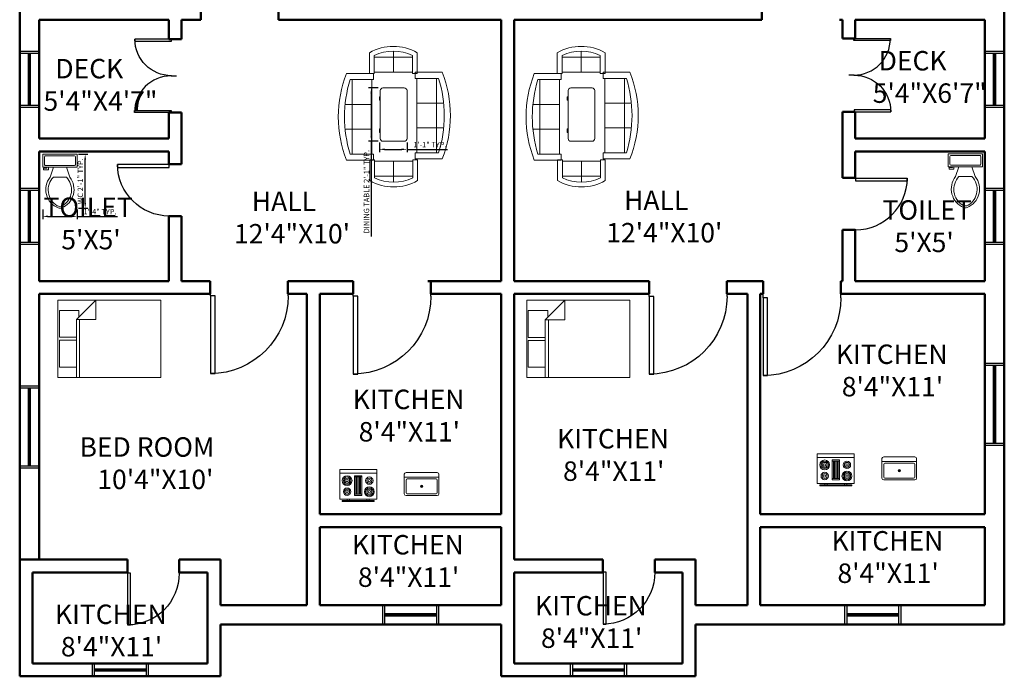
# Model space of a CAD drawing. Units: inches. Extents: x -31438 to -28352, y 12489 to 13610.
# Tile 4 of 5: x -29143 to -28687, y 12722 to 13026. Entities that reach past the tile are written whole.
import ezdxf

# ---------------------------------------------------------------- set-up
doc = ezdxf.new("R2010")
doc.units = ezdxf.units.IN
for name, color, linetype, lineweight in [('A-ANNO-DIMS', 2, 'Continuous', 18), ('A-AREA-IDEN', 3, 'Continuous', 18), ('A-DOOR', 3, 'Continuous', 25), ('A-FLOR-FIXT', 9, 'Continuous', 18), ('A-FURN', 8, 'Continuous', 18), ('A-GLAZ', 4, 'Continuous', 25), ('A-WALL', 7, 'Continuous', 50)]:
    doc.layers.add(name, color=color, linetype=linetype, lineweight=lineweight)
doc.styles.get("Standard").update_dxf_attribs({"font": 'arial.ttf'})
doc.dimstyles.new('ISO-25', dxfattribs={"dimtxt": 2.5, "dimasz": 2.5, "dimexe": 1.25, "dimexo": 0.625, "dimtad": 1, "dimdec": 0, "dimlunit": 3, "dimtxsty": 'Standard', "dimcen": 2.5, "dimadec": 0, "dimazin": 0, "dimtfac": 1, "dimtdec": 0, "dimtmove": 0, "dimatfit": 3, "dimfxl": 1, "dimarcsym": 0})

# ---------------------------------------------------------------- blocks, each defined once
blk = doc.blocks.new('*U8')
for p, q in [((0, 0), (0, -100)), ((750, 0), (750, -100))]:
    blk.add_line(p, q)
blk.add_lwpolyline([(0, 0), (0, 750), (43.75, 750), (43.75, 0)], close=True)
blk.add_arc((0, 0), 750, 0, 90)
blk = doc.blocks.new('Bed - Queen')
for p, q in [((0, -80.00003), (0, 0)), ((0, 0), (59.99999, 0)), ((59.99999, 0), (59.99999, -80.00003)), ((7.99999, -1.2), (28.79998, -1.2)), ((7.99999, -14.4), (7.99999, -1.2)), ((28.79998, -1.2), (28.79998, -14.4)), ((31.19999, -1.2), (51.99999, -1.2)), ((31.19999, -14.4), (31.19999, -1.2)), ((51.99999, -1.2), (51.99999, -16.4)), ((0, -14.4), (44.8, -14.4)), ((59.99999, -29.6), (44.8, -14.4)), ((44.8, -14.4), (44.8, -29.6)), ((44.8, -16.8), (0, -16.8)), ((51.99999, -16.4), (46.79936, -16.4)), ((44.8, -29.6), (59.99999, -29.6)), ((59.99999, -80.00003), (0, -80.00003))]:
    blk.add_line(p, q)
blk = doc.blocks.new('Desk - 30 x 60 in.')
for p, q in [((-26.999995, 0), (26.999995, 0)), ((-29.999995, -27), (-29.999995, -3)), ((29.999995, -3), (29.999995, -27)), ((26.999995, -30), (-26.999995, -30)), ((-20.000005, -30), (-20.000005, -31)), ((-20.000005, -31), (-16.000005, -31)), ((-16.000005, -31), (-16.000005, -30)), ((15.999995, -31), (15.999995, -30)), ((19.999995, -31), (15.999995, -31)), ((19.999995, -30), (19.999995, -31))]:
    blk.add_line(p, q)
for centre, start, end in [((-26.499995, -3.5), 98.1301, 171.8699), ((26.499995, -3.5), 8.130102, 81.8699), ((-26.499995, -26.5), 188.1301, 261.8699), ((26.499995, -26.5), 278.1301, 351.8699)]:
    blk.add_arc(centre, 3.535534, start, end)
blk = doc.blocks.new('Sofa - Roundback 7 ft.')
for p, q in [((-12.00002, -32.4421), (-12.00003, -6.5971)), ((11.99997, -32.4421), (11.99998, -6.5971)), ((-36.000027, -34), (-36.000027, -11.4696)), ((-35.999844, -13.3819), (35.9998, -13.3819)), ((35.99998, -34), (35.99998, -11.4696)), ((-36.000027, -32.4421), (35.99998, -32.4421))]:
    blk.add_line(p, q)
for points in [[(-36.000027, -34), (-42.000027, -34), (-42.000027, -8)], [(41.99998, -8), (41.99998, -34), (35.99998, -34)]]:
    blk.add_lwpolyline(points)
for centre, radius, start, end in [((0, -114.25), 114.25, 68.43141, 111.5686), ((-0.00001, -127.1968), 121.1968, 72.72033, 107.2797)]:
    blk.add_arc(centre, radius, start, end)
blk = doc.blocks.new('Sofa - Roundback Loveseat 5 ft.')
for p, q in [((-24, -33.99998), (-24, -11.46958)), ((0, -32.44198), (0, -5.99998)), ((24.00004, -33.99998), (24.00004, -11.46958)), ((-23.9998, -13.38178), (23.99986, -13.38178)), ((-24, -32.44198), (24.00004, -32.44198))]:
    blk.add_line(p, q)
for points in [[(-24, -33.99998), (-30, -33.99998), (-30, -7.99998)], [(30.00004, -7.99998), (30.00004, -33.99998), (24.00004, -33.99998)]]:
    blk.add_lwpolyline(points)
for centre, radius, start, end in [((0, -60.24998), 60.24998, 60.13715, 119.8628), ((0, -61.38438), 55.38444, 64.32083, 115.6792)]:
    blk.add_arc(centre, radius, start, end)
blk = doc.blocks.new('Toilet - top')
for p, q in [((9.5, -6), (9.5, -2)), ((-10, -8.5), (-8, -8.5)), ((-10, -9.5), (-10, -8.5)), ((-7, -9.5), (-10, -9.5)), ((-8, -8.5), (-8, -8)), ((-7, -8), (-7, -9.5)), ((-4, -8), (-6, -14)), ((4, -8), (6, -14)), ((4, -14), (-4, -14))]:
    blk.add_line(p, q)
blk.add_lwpolyline([(10.5, -8), (10.5, 0), (-10.5, 0), (-10.5, -8)], close=True)
for points in [[(-9.5, -2), (-9.5, -6)], [(8.5, -1), (-8.5, -1)], [(-8.5, -7), (8.5, -7)]]:
    blk.add_lwpolyline(points)
for centre, radius, start, end in [((-8.62, -1.88), 0.884, 81.8699, 188.1301), ((-8.62, -6.12), 0.884, 171.8699, 278.1301), ((8.62, -1.88), 0.884, 351.8699, 98.1301), ((8.62, -6.12), 0.884, 261.8699, 8.1301), ((3.52, -21.58), 12.17, 141.46911, 247.97143), ((4.2, -21.82), 11.33, 136.36773, 238.94682), ((-3.52, -21.58), 12.17, 292.02843, 38.53071), ((-4.2, -21.82), 11.33, 301.05301, 43.63209), ((0, -27.88), 4, 245.73182, 294.26817), ((0, -29), 4, 254.86053, 285.13947)]:
    blk.add_arc(centre, radius, start, end)
blk = doc.blocks.new('Range-Oven - 30 in top')
for p, q in [((0, -3), (30, -3)), ((12, -6), (18, -6)), ((13, -20), (13, -6)), ((14, -6), (14, -20)), ((15, -20), (15, -6)), ((16, -6), (16, -20)), ((17, -20), (17, -6)), ((18, -20), (12, -20)), ((6, -24), (6, -25)), ((8, -25), (8, -24)), ((22, -25), (22, -24)), ((24, -24), (24, -25))]:
    blk.add_line(p, q)
for points in [[(0, -24), (0, 0), (30, 0), (30, -24)], [(12, -21), (12, -5), (18, -5), (18, -21)], [(2, -26), (2, -25), (28, -25), (28, -26)]]:
    blk.add_lwpolyline(points, close=True)
for centre, radius in [((6, -9), 4), ((6, -9), 3), ((6, -9), 2), ((24, -9), 3), ((24, -9), 2), ((6, -18), 3), ((6, -9), 1), ((24, -18), 4), ((24, -18), 3), ((24, -9), 1), ((6, -18), 2), ((6, -18), 1), ((24, -18), 2), ((24, -18), 1)]:
    blk.add_circle(centre, radius)
blk = doc.blocks.new('Sink-single - 30 in top')
blk.add_line((-15, -3.999996), (15, -3.999996))
for points in [[(-13.5, 0), (13.5, 0)], [(-15, -18.499996), (-15, -1.5)], [(-13.5, -17.499996), (-13.5, -6.499996)], [(-12.5, -5.499996), (12.5, -5.499996)], [(13.5, -6.499996), (13.5, -17.499996)], [(15, -1.5), (15, -18.499996)], [(13.5, -19.999996), (-13.5, -19.999996)], [(12.5, -18.499996), (-12.5, -18.499996)]]:
    blk.add_lwpolyline(points)
for radius in [1, 0.5]:
    blk.add_circle((0, -11.999996), radius)
for centre, radius, start, end in [((-13.5, -1.5), 1.5, 90, 180), ((-12.5, -6.499996), 1, 90, 180), ((12.5, -6.499996), 1, 0, 90), ((13.5, -1.5), 1.5, 0, 90), ((-13.5, -18.499996), 1.5, 180, 270), ((-12.5, -17.499996), 1, 180, 270), ((12.5, -17.499996), 1, 270, 0), ((13.5, -18.499996), 1.5, 270, 0)]:
    blk.add_arc(centre, radius, start, end)
blk = doc.blocks.new('WIN-24')
for p, q in [((0, 0), (0, 24)), ((0.5, 0), (0.5, 24))]:
    blk.add_line(p, q)
blk = doc.blocks.new('*D191')
at = {"layer": 'A-ANNO-DIMS', "color": 0, "lineweight": -2, "transparency": 16777216}
for p, q in [((-29115.8, 12963.47), (-29111.42, 12963.47)), ((-29112.67, 12940.94), (-29112.67, 12960.97)), ((-29115.8, 12938.44), (-29111.42, 12938.44))]:
    blk.add_line(p, q, dxfattribs=at)
at = {"layer": 'A-ANNO-DIMS', "color": 0, "transparency": 16777216}
for points in [[(-29113.09, 12960.97), (-29112.25, 12960.97), (-29112.67, 12963.47)], [(-29113.09, 12940.94), (-29112.25, 12940.94), (-29112.67, 12938.44)]]:
    blk.add_solid(points, dxfattribs=at)
at = {"layer": 'Defpoints', "color": 0, "transparency": 16777216}
for p in [(-29116.42, 12963.47), (-29112.67, 12963.47), (-29116.42, 12938.44)]:
    blk.add_point(p, dxfattribs=at)
at = {"layer": 'A-ANNO-DIMS', "color": 0, "transparency": 16777216, "insert": (-29114.59, 12950.96), "char_height": 2.5, "attachment_point": 5, "rotation": 90}
blk.add_mtext('WC 2\'-1" TYP.', dxfattribs=at)
blk = doc.blocks.new('*D192')
at = {"layer": 'A-ANNO-DIMS', "color": 0, "lineweight": -2, "transparency": 16777216}
for p, q in [((-29132.33, 12937.81), (-29132.33, 12933.43)), ((-29116.42, 12937.81), (-29116.42, 12933.43)), ((-29129.83, 12934.68), (-29118.92, 12934.68)), ((-29116.42, 12934.68), (-29097.67, 12934.68))]:
    blk.add_line(p, q, dxfattribs=at)
at = {"layer": 'A-ANNO-DIMS', "color": 0, "transparency": 16777216}
for points in [[(-29129.83, 12935.1), (-29129.83, 12934.27), (-29132.33, 12934.68)], [(-29118.92, 12935.1), (-29118.92, 12934.27), (-29116.42, 12934.68)]]:
    blk.add_solid(points, dxfattribs=at)
at = {"layer": 'Defpoints', "color": 0, "transparency": 16777216}
for p in [(-29132.33, 12938.44), (-29116.42, 12938.44), (-29116.42, 12934.68)]:
    blk.add_point(p, dxfattribs=at)
at = {"layer": 'A-ANNO-DIMS', "color": 0, "transparency": 16777216, "insert": (-29105.8, 12936.56), "char_height": 2.5, "attachment_point": 5}
blk.add_mtext('1\'-4" TYP.', dxfattribs=at)
blk = doc.blocks.new('*D203')
at = {"layer": 'A-ANNO-DIMS', "color": 0, "lineweight": -2, "transparency": 16777216}
for p, q in [((-28977.05, 12994.22), (-28981.39, 12994.22)), ((-28980.14, 12991.72), (-28980.14, 12971.94)), ((-28977.05, 12969.44), (-28981.39, 12969.44)), ((-28980.14, 12969.44), (-28980.14, 12925.35))]:
    blk.add_line(p, q, dxfattribs=at)
at = {"layer": 'A-ANNO-DIMS', "color": 0, "transparency": 16777216}
for points in [[(-28980.56, 12991.72), (-28979.72, 12991.72), (-28980.14, 12994.22)], [(-28980.56, 12971.94), (-28979.72, 12971.94), (-28980.14, 12969.44)]]:
    blk.add_solid(points, dxfattribs=at)
at = {"layer": 'Defpoints', "color": 0, "transparency": 16777216}
for p in [(-28976.42, 12994.22), (-28980.14, 12969.44), (-28976.42, 12969.44)]:
    blk.add_point(p, dxfattribs=at)
at = {"layer": 'A-ANNO-DIMS', "color": 0, "transparency": 16777216, "insert": (-28982.06, 12946.15), "char_height": 2.5, "attachment_point": 5, "rotation": 90}
blk.add_mtext('DINING TABLE 2\'-1" TYP.', dxfattribs=at)
blk = doc.blocks.new('*D204')
at = {"layer": 'A-ANNO-DIMS', "color": 0, "lineweight": -2, "transparency": 16777216}
for p, q in [((-28976.42, 12968.82), (-28976.42, 12964.47)), ((-28963.62, 12968.82), (-28963.62, 12964.47)), ((-28973.92, 12965.72), (-28966.12, 12965.72)), ((-28963.62, 12965.72), (-28944.87, 12965.72))]:
    blk.add_line(p, q, dxfattribs=at)
at = {"layer": 'A-ANNO-DIMS', "color": 0, "transparency": 16777216}
for points in [[(-28973.92, 12966.14), (-28973.92, 12965.31), (-28976.42, 12965.72)], [(-28966.12, 12966.14), (-28966.12, 12965.31), (-28963.62, 12965.72)]]:
    blk.add_solid(points, dxfattribs=at)
at = {"layer": 'Defpoints', "color": 0, "transparency": 16777216}
for p in [(-28976.42, 12969.44), (-28963.62, 12969.44), (-28963.62, 12965.72)]:
    blk.add_point(p, dxfattribs=at)
at = {"layer": 'A-ANNO-DIMS', "color": 0, "transparency": 16777216, "insert": (-28952.99, 12967.61), "char_height": 2.5, "attachment_point": 5}
blk.add_mtext('1\'-1" TYP.', dxfattribs=at)

msp = doc.modelspace()

# ---------------------------------------------------------------- linework, layer by layer
at = {"layer": 'A-GLAZ'}
for p, q in [((-29142.99, 13011.25), (-29133.99, 13011.25)), ((-29142.99, 13010.25), (-29133.99, 13010.25)), ((-29138.99, 12986.25), (-29138.99, 13010.25)), ((-29138.49, 12986.25), (-29138.49, 13010.25)), ((-29137.99, 12986.25), (-29137.99, 13010.25)), ((-28695.99, 13011.25), (-28686.99, 13011.25)), ((-28695.99, 13010.25), (-28686.99, 13010.25)), ((-28691.99, 12986.25), (-28691.99, 13010.25)), ((-28691.49, 12986.25), (-28691.49, 13010.25)), ((-28690.99, 12986.25), (-28690.99, 13010.25)), ((-29142.99, 12986.25), (-29133.99, 12986.25)), ((-29142.99, 12985.25), (-29133.99, 12985.25)), ((-28695.99, 12986.25), (-28686.99, 12986.25)), ((-28695.99, 12985.25), (-28686.99, 12985.25)), ((-29142.99, 12947.75), (-29133.99, 12947.75)), ((-29142.99, 12946.75), (-29133.99, 12946.75)), ((-29138.99, 12922.75), (-29138.99, 12946.75)), ((-29138.49, 12922.75), (-29138.49, 12946.75)), ((-29137.99, 12922.75), (-29137.99, 12946.75)), ((-28695.99, 12947.75), (-28686.99, 12947.75)), ((-28695.99, 12946.75), (-28686.99, 12946.75)), ((-28691.99, 12922.75), (-28691.99, 12946.75)), ((-28691.49, 12922.75), (-28691.49, 12946.75)), ((-28690.99, 12922.75), (-28690.99, 12946.75)), ((-29142.99, 12922.75), (-29133.99, 12922.75)), ((-29142.99, 12921.75), (-29133.99, 12921.75)), ((-28695.99, 12922.75), (-28686.99, 12922.75)), ((-28695.99, 12921.75), (-28686.99, 12921.75)), ((-28695.99, 12866.75), (-28686.99, 12866.75)), ((-28695.99, 12865.75), (-28686.99, 12865.75)), ((-28691.99, 12829.75), (-28691.99, 12865.75)), ((-28691.49, 12829.75), (-28691.49, 12865.75)), ((-28690.99, 12829.75), (-28690.99, 12865.75)), ((-29142.99, 12856.25), (-29133.99, 12856.25)), ((-29142.99, 12855.25), (-29133.99, 12855.25)), ((-29138.99, 12819.25), (-29138.99, 12855.25)), ((-29138.49, 12819.25), (-29138.49, 12855.25)), ((-29137.99, 12819.25), (-29137.99, 12855.25)), ((-28695.99, 12829.75), (-28686.99, 12829.75)), ((-28695.99, 12828.75), (-28686.99, 12828.75)), ((-29142.99, 12819.25), (-29133.99, 12819.25)), ((-29142.99, 12818.25), (-29133.99, 12818.25)), ((-28974.99, 12754.75), (-28974.99, 12745.75)), ((-28973.99, 12754.75), (-28973.99, 12745.75)), ((-28949.99, 12754.75), (-28949.99, 12745.75)), ((-28948.99, 12754.75), (-28948.99, 12745.75)), ((-28760.99, 12754.75), (-28760.99, 12745.75)), ((-28759.99, 12754.75), (-28759.99, 12745.75)), ((-28735.99, 12754.75), (-28735.99, 12745.75)), ((-28734.99, 12754.75), (-28734.99, 12745.75)), ((-28973.99, 12750.75), (-28949.99, 12750.75)), ((-28759.99, 12750.75), (-28735.99, 12750.75)), ((-29109.49, 12727.75), (-29109.49, 12721.75)), ((-29108.49, 12727.75), (-29108.49, 12721.75)), ((-29084.49, 12727.75), (-29084.49, 12721.75)), ((-29083.49, 12727.75), (-29083.49, 12721.75)), ((-28887.99, 12727.75), (-28887.99, 12721.75)), ((-28886.99, 12727.75), (-28886.99, 12721.75)), ((-28862.99, 12727.75), (-28862.99, 12721.75)), ((-28861.99, 12727.75), (-28861.99, 12721.75)), ((-29108.49, 12725.25), (-29084.49, 12725.25)), ((-29108.49, 12724.75), (-29084.49, 12724.75)), ((-29108.49, 12724.25), (-29084.49, 12724.25)), ((-28886.99, 12725.25), (-28862.99, 12725.25)), ((-28886.99, 12724.75), (-28862.99, 12724.75)), ((-28886.99, 12724.25), (-28862.99, 12724.25))]:
    msp.add_line(p, q, dxfattribs=at)
at = {"layer": 'A-WALL'}
for p, q in [((-28686.99, 13609.75), (-28686.99, 12745.75)), ((-29142.99, 12721.75), (-29142.99, 13585.75)), ((-29059.11, 13031.75), (-29059.11, 13025.75)), ((-29023.11, 13031.75), (-29023.11, 13025.75)), ((-28799.32, 13031.75), (-28799.32, 13025.75)), ((-29073.99, 13025.75), (-29133.99, 13025.75)), ((-29133.99, 12970.75), (-29133.99, 13025.75)), ((-29073.99, 13016.72), (-29073.99, 13025.75)), ((-29059.11, 13025.75), (-29067.99, 13025.75)), ((-29067.99, 13016.72), (-29067.99, 13025.75)), ((-28953.99, 13025.75), (-29023.11, 13025.75)), ((-28919.99, 13025.75), (-28953.99, 13025.75)), ((-28919.99, 12904.75), (-28919.99, 13025.75)), ((-28799.32, 13025.75), (-28913.99, 13025.75)), ((-28913.99, 12904.75), (-28913.99, 13025.75)), ((-28761.99, 13025.75), (-28763.32, 13025.75)), ((-28761.99, 13025.75), (-28761.99, 13017.05)), ((-28755.99, 13025.75), (-28755.99, 13017.05)), ((-28695.99, 13025.75), (-28755.99, 13025.75)), ((-28695.99, 13025.75), (-28755.99, 13025.75)), ((-28695.99, 13025.75), (-28695.99, 12970.75)), ((-29073.99, 13016.72), (-29067.99, 13016.72)), ((-28761.99, 13017.05), (-28755.99, 13017.05)), ((-29073.99, 12970.75), (-29073.99, 12982.72)), ((-29073.99, 12982.72), (-29067.99, 12982.72)), ((-29067.99, 12958.83), (-29067.99, 12982.72)), ((-28761.99, 12983.05), (-28761.99, 12952.5)), ((-28761.99, 12983.05), (-28755.99, 12983.05)), ((-28755.99, 12983.05), (-28755.99, 12970.75)), ((-29073.99, 12970.75), (-29133.99, 12970.75)), ((-28695.99, 12970.75), (-28755.99, 12970.75)), ((-28695.99, 12970.75), (-28755.99, 12970.75)), ((-29073.99, 12964.75), (-29133.99, 12964.75)), ((-29133.99, 12904.75), (-29133.99, 12964.75)), ((-29073.99, 12958.83), (-29073.99, 12964.75)), ((-28755.99, 12964.75), (-28755.99, 12952.5)), ((-28695.99, 12964.75), (-28755.99, 12964.75)), ((-28695.99, 12964.75), (-28755.99, 12964.75)), ((-28695.99, 12964.75), (-28695.99, 12904.75)), ((-29073.99, 12958.83), (-29067.99, 12958.83)), ((-28761.99, 12952.5), (-28755.99, 12952.5)), ((-29073.99, 12904.75), (-29073.99, 12934.83)), ((-29073.99, 12934.83), (-29067.99, 12934.83)), ((-29067.99, 12904.75), (-29067.99, 12934.83)), ((-28761.99, 12928.5), (-28761.99, 12904.75)), ((-28761.99, 12928.5), (-28755.99, 12928.5)), ((-28755.99, 12928.5), (-28755.99, 12904.75)), ((-29073.99, 12904.75), (-29133.99, 12904.75)), ((-29054.81, 12904.75), (-29067.99, 12904.75)), ((-29054.81, 12904.75), (-29054.81, 12898.75)), ((-28988.61, 12904.75), (-29018.81, 12904.75)), ((-29018.81, 12904.75), (-29018.81, 12898.75)), ((-28988.61, 12904.75), (-28988.61, 12898.75)), ((-28919.99, 12904.75), (-28953.99, 12904.75)), ((-28952.61, 12904.75), (-28952.61, 12898.75)), ((-28851.47, 12904.75), (-28913.99, 12904.75)), ((-28851.47, 12904.75), (-28851.47, 12898.75)), ((-28798.69, 12904.75), (-28815.47, 12904.75)), ((-28815.47, 12904.75), (-28815.47, 12898.75)), ((-28798.69, 12898.75), (-28798.69, 12904.75)), ((-28761.99, 12904.75), (-28762.69, 12904.75)), ((-28762.69, 12898.75), (-28762.69, 12904.75)), ((-28695.99, 12904.75), (-28755.99, 12904.75)), ((-29054.81, 12898.75), (-29133.99, 12898.75)), ((-29133.99, 12775.75), (-29133.99, 12898.75)), ((-29009.99, 12898.75), (-29018.81, 12898.75)), ((-29009.99, 12754.75), (-29009.99, 12898.75)), ((-28988.61, 12898.75), (-29003.99, 12898.75)), ((-29003.99, 12796.75), (-29003.99, 12898.75)), ((-28919.99, 12898.75), (-28952.61, 12898.75)), ((-28919.99, 12796.75), (-28919.99, 12898.75)), ((-28851.47, 12898.75), (-28913.99, 12898.75)), ((-28913.99, 12775.75), (-28913.99, 12898.75)), ((-28805.99, 12898.75), (-28815.47, 12898.75)), ((-28805.99, 12754.75), (-28805.99, 12898.75)), ((-28798.69, 12898.75), (-28799.99, 12898.75)), ((-28799.99, 12796.75), (-28799.99, 12898.75)), ((-28695.99, 12898.75), (-28762.69, 12898.75)), ((-28695.99, 12898.75), (-28695.99, 12796.75)), ((-28919.99, 12796.75), (-29003.99, 12796.75)), ((-28695.99, 12796.75), (-28799.99, 12796.75)), ((-28919.99, 12790.75), (-29003.99, 12790.75)), ((-29003.99, 12754.75), (-29003.99, 12790.75)), ((-28919.99, 12754.75), (-28919.99, 12790.75)), ((-28695.99, 12790.75), (-28799.99, 12790.75)), ((-28799.99, 12754.75), (-28799.99, 12790.75)), ((-28695.99, 12790.75), (-28695.99, 12754.75)), ((-29093.09, 12775.75), (-29142.99, 12775.75)), ((-29093.09, 12775.75), (-29093.09, 12769.75)), ((-29049.99, 12775.75), (-29069.09, 12775.75)), ((-29069.09, 12775.75), (-29069.09, 12769.75)), ((-29049.99, 12754.75), (-29049.99, 12775.75)), ((-28872.86, 12775.75), (-28913.99, 12775.75)), ((-28872.86, 12775.75), (-28872.86, 12769.75)), ((-28829.99, 12775.75), (-28848.86, 12775.75)), ((-28848.86, 12775.75), (-28848.86, 12769.75)), ((-28829.99, 12754.75), (-28829.99, 12775.75)), ((-29093.09, 12769.75), (-29136.99, 12769.75)), ((-29136.99, 12727.75), (-29136.99, 12769.75)), ((-29055.99, 12769.75), (-29069.09, 12769.75)), ((-29055.99, 12727.75), (-29055.99, 12769.75)), ((-28872.86, 12769.75), (-28913.99, 12769.75)), ((-28913.99, 12727.75), (-28913.99, 12769.75)), ((-28835.99, 12769.75), (-28848.86, 12769.75)), ((-28835.99, 12727.75), (-28835.99, 12769.75)), ((-29009.99, 12754.75), (-29049.99, 12754.75)), ((-28919.99, 12754.75), (-29003.99, 12754.75)), ((-28805.99, 12754.75), (-28829.99, 12754.75)), ((-28695.99, 12754.75), (-28799.99, 12754.75)), ((-28919.99, 12745.75), (-29049.99, 12745.75)), ((-29049.99, 12721.75), (-29049.99, 12745.75)), ((-28919.99, 12721.75), (-28919.99, 12745.75)), ((-28686.99, 12745.75), (-28829.99, 12745.75)), ((-28829.99, 12721.75), (-28829.99, 12745.75)), ((-29055.99, 12727.75), (-29136.99, 12727.75)), ((-28835.99, 12727.75), (-28913.99, 12727.75)), ((-29049.99, 12721.75), (-29142.99, 12721.75)), ((-28829.99, 12721.75), (-28919.99, 12721.75))]:
    msp.add_line(p, q, dxfattribs=at)

# ---------------------------------------------------------------- block references
at = {"layer": 'A-DOOR'}
for p, xscale, yscale, zscale, rotation in [((-29072.66, 13016.78), -0.022636277250161, 0.022636277250161, 0.022636277250161, 90), ((-28756.73, 13017.06), 0.022636277250161, 0.022636277250161, 0.022636277250161, 270), ((-29072.83, 12982.76), 0.022666666666667, 0.022666666666667, 0.022666666666667, 90.00000000000003), ((-28756.57, 12983.05), -0.022666666666667, 0.022666666666667, 0.022666666666667, 270), ((-29073.77, 12958.75), -0.031855356978981, 0.031855356978981, 0.031855356978981, 90), ((-28755.81, 12952.39), 0.031855356978981, 0.031855356978981, 0.031855356978981, 270), ((-29054.62, 12897.9), -0.0480000000000062, 0.0480000000000062, 0.0480000000000062, 180), ((-28988.56, 12897.71), -0.0480000000000062, 0.0480000000000062, 0.0480000000000062, 180), ((-28851.41, 12897.66), -0.0480000000000062, 0.0480000000000062, 0.0480000000000062, 180), ((-28798.69, 12896.95), -0.0480000000000062, 0.0480000000000062, 0.0480000000000062, 180), ((-29093.12, 12769.53), -0.0320000000000025, 0.0320000000000025, 0.0320000000000025, 180), ((-28872.81, 12769.91), -0.0320000000000025, 0.0320000000000025, 0.0320000000000025, 180)]:
    msp.add_blockref('*U8', p, dxfattribs=dict(at, xscale=xscale, yscale=yscale, zscale=zscale, rotation=rotation))
at = {"layer": 'A-FLOR-FIXT'}
for name, p, xscale, yscale, zscale in [('Toilet - top', (-29124.38, 12963.47), 0.7575755229467699, 0.7575755229467699, 0.7575755229467699), ('Toilet - top', (-28704.99, 12963.69), 0.7575755229467699, 0.7575755229467699, 0.7575755229467699), ('Range-Oven - 30 in top', (-28773.6, 12824.76), 0.5716393668778607, 0.5716393668778607, 0.5716393668778607), ('Sink-single - 30 in top', (-28735.65, 12823.36), 0.534256555286997, 0.534256555286997, 0.534256555286997), ('Range-Oven - 30 in top', (-28994.8, 12817.49), 0.5716393668778607, 0.5716393668778607, 0.5716393668778607), ('Sink-single - 30 in top', (-28956.85, 12816.09), 0.534256555286997, 0.534256555286997, 0.534256555286997)]:
    msp.add_blockref(name, p, dxfattribs=dict(at, xscale=xscale, yscale=yscale, zscale=zscale))
at = {"layer": 'A-FURN', "xscale": 0.3682442798772706, "yscale": 0.3682442798772706, "zscale": 0.3682442798772706}
for p in [(-28969.93, 13013.39), (-28882.96, 13013.39)]:
    msp.add_blockref('Sofa - Roundback Loveseat 5 ft.', p, dxfattribs=at)
at = {"layer": 'A-FURN'}
for name, p, xscale, yscale, zscale, rotation in [('Sofa - Roundback 7 ft.', (-28995.45, 12980.78), 0.4784035434924597, 0.4784035434924597, 0.4784035434924597, 89.99999999999999), ('Sofa - Roundback 7 ft.', (-28943.51, 12981.35), 0.4784035434924597, 0.4784035434924597, 0.4784035434924597, 270), ('Sofa - Roundback 7 ft.', (-28908.48, 12980.78), 0.4784035434924597, 0.4784035434924597, 0.4784035434924597, 89.99999999999999), ('Sofa - Roundback 7 ft.', (-28856.54, 12981.35), 0.4784035434924597, 0.4784035434924597, 0.4784035434924597, 270), ('Desk - 30 x 60 in.', (-28963.62, 12981.83), 0.4130441003592061, 0.4130441003592061, 0.4130441003592061, 270), ('Desk - 30 x 60 in.', (-28876.65, 12981.83), 0.4130441003592061, 0.4130441003592061, 0.4130441003592061, 270), ('Sofa - Roundback Loveseat 5 ft.', (-28969.8, 12948.32), 0.3682442798772706, 0.3682442798772706, 0.3682442798772706, 180), ('Sofa - Roundback Loveseat 5 ft.', (-28882.83, 12948.32), 0.3682442798772706, 0.3682442798772706, 0.3682442798772706, 180), ('Bed - Queen', (-29125.34, 12860.12), 0.597358992664269, 0.597358992664269, 0.597358992664269, 90), ('Bed - Queen', (-28908.18, 12860.02), 0.597358992664269, 0.597358992664269, 0.597358992664269, 90)]:
    msp.add_blockref(name, p, dxfattribs=dict(at, xscale=xscale, yscale=yscale, zscale=zscale, rotation=rotation))
at = {"layer": 'A-GLAZ'}
for p, rotation in [((-28973.99, 12750.25), 270.0000000000004), ((-28759.99, 12750.25), 270.0000000000007)]:
    msp.add_blockref('WIN-24', p, dxfattribs=dict(at, rotation=rotation))

# ---------------------------------------------------------------- texts
at = {"layer": 'A-AREA-IDEN', "char_height": 9, "attachment_point": 1}
for s, insert in [('{  DECK\\P 5\'4"X6\'7"}', (-28750.68, 13011.25)), ('{  DECK\\P5\'4"X4\'7"}', (-29131.97, 13007.58)), ('{   HALL\\P12\'4"X10\'}', (-29043.74, 12946.15)), ('{   HALL\\P12\'4"X10\'}', (-28871.33, 12946.63)), ("{TOILET\\P   5'X5'}", (-29131.97, 12943.42)), ("{  TOILET\\P    5'X5'}", (-28748.89, 12942.14)), ('{KITCHEN\\P 8\'4"X11\'}', (-28765, 12875.36)), ('{KITCHEN\\P 8\'4"X11\'}', (-28988.76, 12854.46)), ('{KITCHEN\\P 8\'4"X11\'}', (-28894.1, 12836.24)), ('{BED ROOM\\P   10\'4"X10\'}', (-29115.28, 12832.41)), ('{KITCHEN\\P 8\'4"X11\'}', (-28989.1, 12787.16)), ('{KITCHEN\\P 8\'4"X11\'}', (-28767.02, 12788.98)), ('{KITCHEN\\P 8\'4"X11\'}', (-28904.32, 12758.91)), ('{KITCHEN\\P 8\'4"X11\'}', (-29126.66, 12754.96))]:
    msp.add_mtext_dynamic_manual_height_columns(s, width=772.4312, gutter_width=12.5, heights=[0], dxfattribs=dict(at, insert=insert))

# ---------------------------------------------------------------- dimensions: what is measured, and where the dimension line sits
at = {"layer": 'A-ANNO-DIMS'}
for base, p1, p2, angle, text, picture, middle in [((-28980.14, 12969.44), (-28976.42, 12994.22), (-28976.42, 12969.44), 270, 'DINING TABLE <> TYP.', '*D203', (-28982.06, 12946.15)), ((-29112.67, 12963.47), (-29116.42, 12938.44), (-29116.42, 12963.47), 90, 'WC <> TYP.', '*D191', (-29114.59, 12950.96))]:
    dim = msp.add_linear_dim(base=base, p1=p1, p2=p2, angle=angle, text=text, dimstyle='ISO-25', override={"dimdec": 1, "dimlfac": 1, "dimrnd": 0, "dimzin": 1, "dimdsep": 46, "dimlunit": 4, "dimfrac": 2}, dxfattribs=at)
    dim.commit()
    dim.dimension.update_dxf_attribs({"geometry": picture, "text_midpoint": middle})
for base, p1, p2, picture, middle in [((-28963.62, 12965.72), (-28976.42, 12969.44), (-28963.62, 12969.44), '*D204', (-28952.99, 12967.61)), ((-29116.42, 12934.68), (-29132.33, 12938.44), (-29116.42, 12938.44), '*D192', (-29105.8, 12936.56))]:
    dim = msp.add_linear_dim(base=base, p1=p1, p2=p2, text='<> TYP.', dimstyle='ISO-25', override={"dimdec": 1, "dimlfac": 1, "dimrnd": 0, "dimzin": 1, "dimdsep": 46, "dimlunit": 4, "dimfrac": 2}, dxfattribs=at)
    dim.commit()
    dim.dimension.update_dxf_attribs({"geometry": picture, "text_midpoint": middle})

doc.saveas('drawing.dxf')
